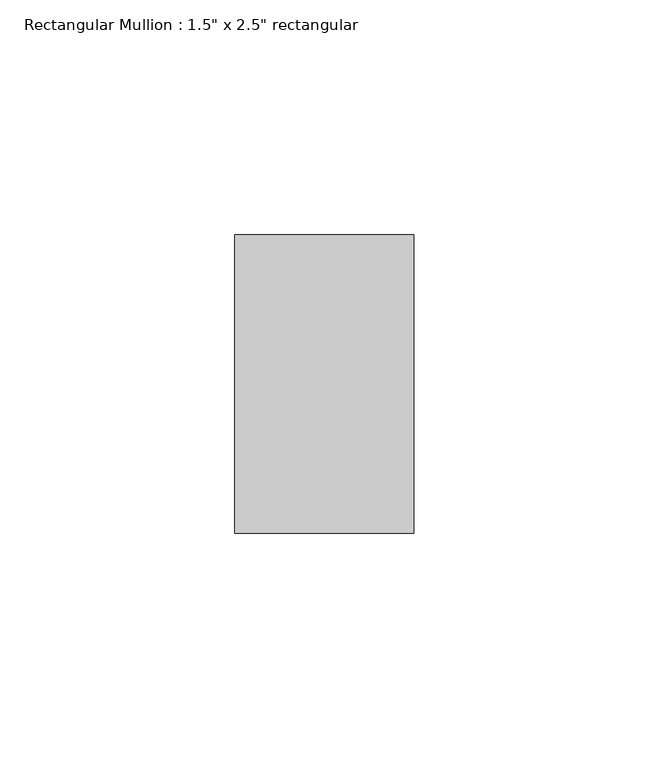
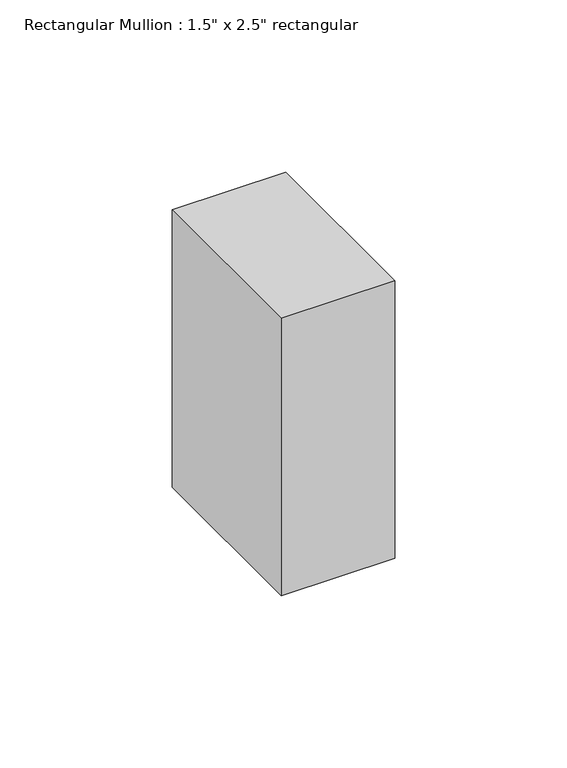
"""IFC4 building model written with IfcOpenShell, lengths in millimetres: member geometry."""

from ifc_helpers import new_model, si_unit, frame, origin, place, context, project, spatial, polyline, outline, extrude, source, transform, mapped, element, save


def member_fdc2508a(model_context):
    return source(origin(), model_context, "Body", "SweptSolid", [
        extrude(outline(polyline([(0.0, 31.75), (0.0, -31.75), (-38.1, -31.75), (-38.1, 31.75), (0.0, 31.75)])), frame((0.0, 0.0, -98.6074046), z_axis=(0.0, 0.0, 1.0), x_axis=(1.0, 0.0, 0.0)), (0.0, 0.0, 1.0), 98.6074046),
    ])


if __name__ == "__main__":
    model = new_model("IFC4")
    model_context = context("Model", 3, world=origin())
    ifc_project = project(units=[si_unit("LENGTHUNIT", "METRE", prefix="MILLI")], contexts=[model_context])
    site = spatial("IfcSite", under=ifc_project)
    building = spatial("IfcBuilding", under=site)
    placement = place(None, origin())
    member_shape = member_fdc2508a(model_context)
    element("IfcMember", 1, ObjectType="Rectangular Mullion : 1.5\" x 2.5\" rectangular", at=placement, inside=building, context=model_context, shape_type="MappedRepresentation", body=[
        mapped(member_shape, transform((0.0, 0.0, 0.0), x_axis=(1.0, 0.0, 0.0), y_axis=(0.0, 1.0, 0.0), z_axis=(0.0, 0.0, 1.0))),
    ])
    save(model, "model.ifc")

# Revit data of these elements
# Type "Rectangular Mullion : 1.5\" x 2.5\" rectangular"
#   built-in parameter 1007304 = 0.208333 (stored number, unit not read)
#   built-in parameter 1007301 = 0.0625 (stored number, unit not read)
#   built-in parameter 1007300 = 0.0625 (stored number, unit not read)
